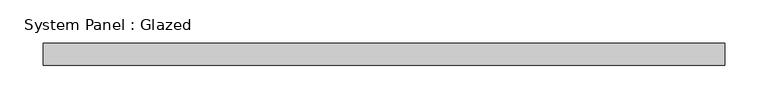
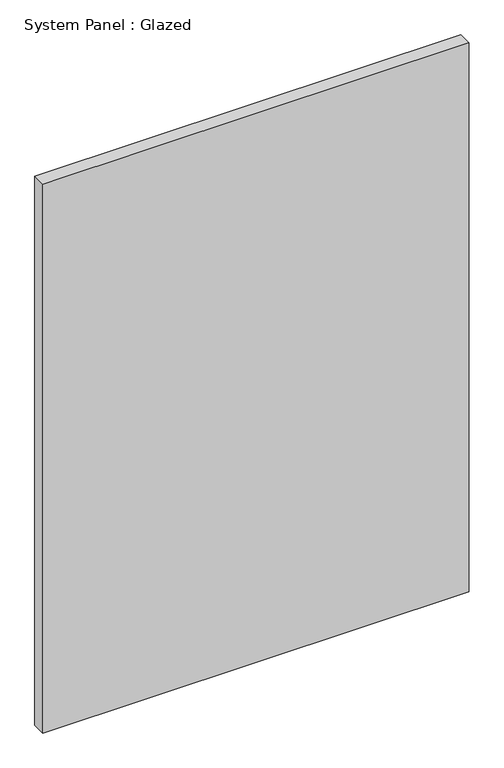
"""IFC4 building model written with IfcOpenShell, lengths in millimetres: plate geometry, System Panel : Glazed."""

from ifc_helpers import new_model, si_unit, origin, origin_with_axes, place, context, project, spatial, polyline, outline, extrude, source, transform, mapped, element, save


def system_panel_glazed_0c055d28(model_context):
    return source(origin(), model_context, "Body", "SweptSolid", [
        extrude(outline(polyline([(394.3296124, 19.05), (-394.3296124, 19.05), (-394.3296124, 44.45), (394.3296124, 44.45), (394.3296124, 19.05)])), origin_with_axes(), (0.0, 0.0, 1.0), 1073.15),
    ])


if __name__ == "__main__":
    model = new_model("IFC4")
    model_context = context("Model", 3, world=origin())
    ifc_project = project(units=[si_unit("LENGTHUNIT", "METRE", prefix="MILLI")], contexts=[model_context])
    site = spatial("IfcSite", under=ifc_project)
    building = spatial("IfcBuilding", under=site)
    placement = place(None, origin())
    system_panel_glazed_shape = system_panel_glazed_0c055d28(model_context)
    element("IfcPlate", 1, ObjectType="System Panel : Glazed", at=placement, inside=building, context=model_context, shape_type="MappedRepresentation", body=[
        mapped(system_panel_glazed_shape, transform((0.0, 0.0, 0.0), x_axis=(1.0, 0.0, 0.0), y_axis=(0.0, 1.0, 0.0), z_axis=(0.0, 0.0, 1.0))),
    ])
    save(model, "model.ifc")

# Revit data of these elements
# Type "System Panel : Glazed"
#   Construction Type Id = "GSP4R"
#   Analytic Construction = "1/8 in Pilkington single glazing"
#   Visual Light Transmittance = 0.9
#   Solar Heat Gain Coefficient = 0.86
#   Heat Transfer Coefficient (U) = 1.18115 BTU/(h·ft²·°F)
# Element 1 (IfcPlate, "System Panel : Glazed")
#   Materials on its faces: "Glass"
# Materials
#   "Glass": class "Glass", colour RGB 0 128 192, transparency 0.75, Description = "Soda Lime Glass", Cost = 0
